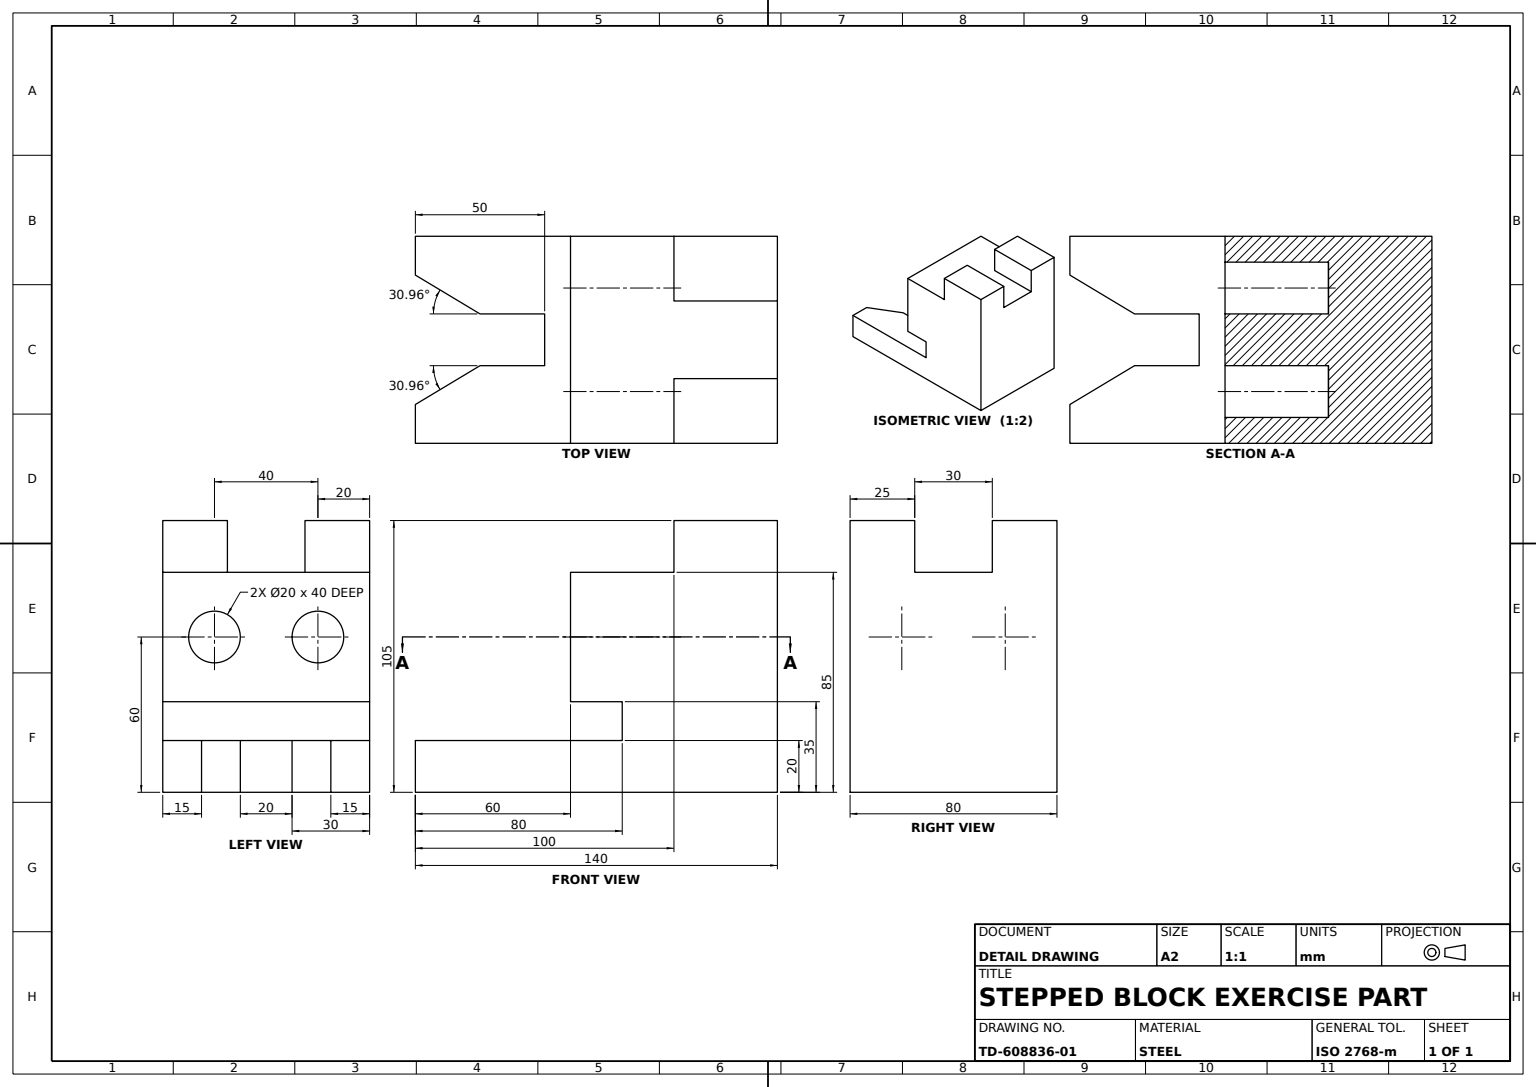
from build123d import *

# Parameters (mm, degrees)
BASE_STEP_BODY_DEPTH        = 80
UPPER_BLOCK_SKETCH_W        = 40
UPPER_BLOCK_SKETCH_H        = 20
UPPER_BLOCK_DEPTH           = 80
CORNER_NOTCH_SKETCH_25X25_W = 40
CORNER_NOTCH_SKETCH_25X25_H = 30
CORNER_NOTCH_25X25_DEPTH    = 20
SIDE_RECESS_DEPTH           = 183.277261336
SIDE_RECESS_DEPTH_BACK      = 20
SLOT_SKETCH_R               = 10
SLOT_CUT_DEPTH              = 40


with BuildPart() as part:
    # Base Step Profile Sketch → Base Step Body (new body)
    with BuildSketch(Plane.XY):
        Polygon((0, 0), (140, 0), (140, 80), (140, 85), (60, 85), (60, 35), (80, 35), (80, 20), (0, 20), align=None)
    extrude(amount=BASE_STEP_BODY_DEPTH)

    # Upper Block Sketch → Upper Block (add)
    with BuildSketch(Plane.XY.offset(80)):
        with Locations((120, 95)):
            Rectangle(UPPER_BLOCK_SKETCH_W, UPPER_BLOCK_SKETCH_H)
    extrude(amount=-UPPER_BLOCK_DEPTH)

    # Corner Notch Sketch 25x25 → Corner Notch 25x25 (cut)
    with BuildSketch(Plane(origin=(0, 105, 0), x_dir=(1, 0, 0), z_dir=(0, 1, 0))):
        with Locations((120, -40)):
            Rectangle(CORNER_NOTCH_SKETCH_25X25_W, CORNER_NOTCH_SKETCH_25X25_H)
    extrude(amount=-CORNER_NOTCH_25X25_DEPTH, mode=Mode.SUBTRACT)

    # Side Recess Sketch → Side Recess (cut, two sides: drawn at the far end of the back side and taken through both)
    with BuildSketch(Plane(origin=(0, 20, 0), x_dir=(1, 0, 0), z_dir=(0, 1, 0)).offset(-SIDE_RECESS_DEPTH_BACK)):
        Polygon((25, -30), (0, -15), (0, -65), (25, -50), (50, -50), (50, -40), (50, -30), align=None)
    extrude(amount=SIDE_RECESS_DEPTH + SIDE_RECESS_DEPTH_BACK, mode=Mode.SUBTRACT)

    # Slot Sketch → Slot Cut (cut)
    with BuildSketch(Plane.ZY.offset(-60)):
        with Locations((20, 60)):
            Circle(SLOT_SKETCH_R)
        with Locations((60, 60)):
            Circle(SLOT_SKETCH_R)
    extrude(amount=-SLOT_CUT_DEPTH, mode=Mode.SUBTRACT)


solid = part.part
